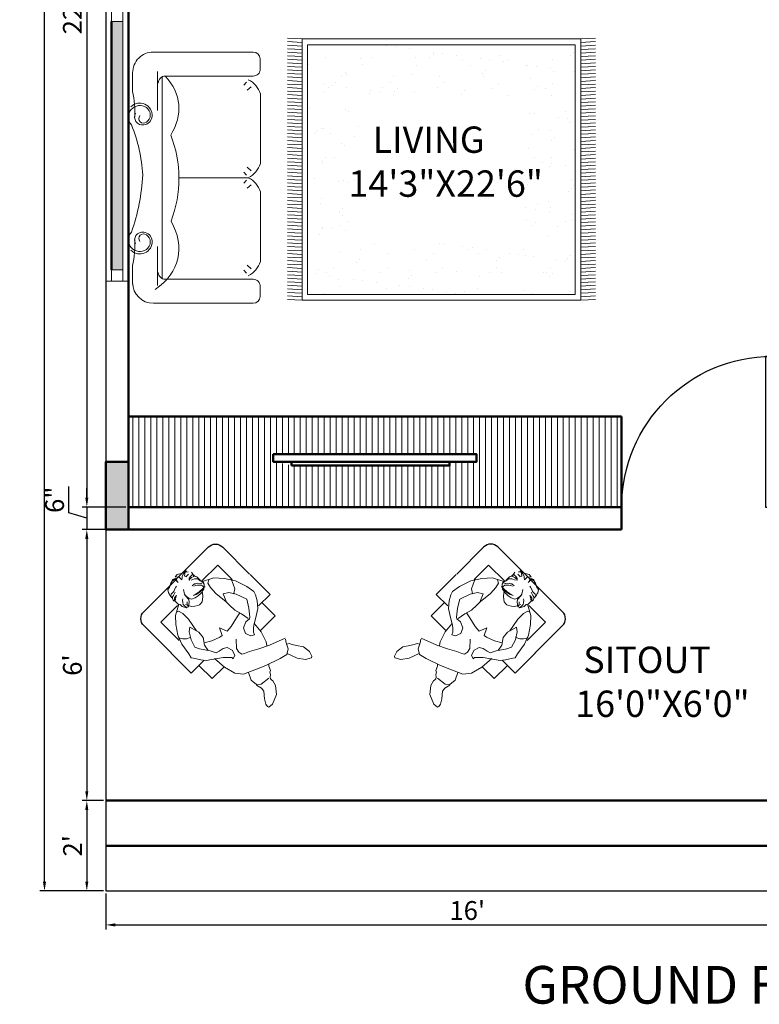
# Model space of a CAD drawing. Units: inches. Extents: x 3064 to 19385, y 846 to 15425.
# Tile 26 of 108: x 4742 to 4938, y 846 to 1108. Entities that reach past the tile are written whole.
import ezdxf

# ---------------------------------------------------------------- set-up
doc = ezdxf.new("R2010")
doc.units = ezdxf.units.IN
for name, color, linetype, lineweight in [('A-ANNO-DIMS', 2, 'Continuous', 18), ('A-ANNO-TEXT', 7, 'Continuous', 25), ('A-AREA-IDEN', 3, 'Continuous', 18), ('A-COLS', 1, 'Continuous', 35), ('A-DOOR', 3, 'Continuous', 25), ('A-FURN', 8, 'Continuous', 18), ('A-FURN-PATT', 252, 'Continuous', 13), ('A-GLAZ', 4, 'Continuous', 18), ('A-WALL', 7, 'Continuous', 50), ('C-PROP', 6, 'Continuous', 25)]:
    doc.layers.add(name, color=color, linetype=linetype, lineweight=lineweight)
doc.layers.add('NOITHAT', color=21, linetype='Continuous')
doc.styles.get("Standard").update_dxf_attribs({"font": 'arial.ttf'})
doc.dimstyles.new('ISO-25', dxfattribs={"dimtxt": 9, "dimasz": 2.5, "dimexe": 1.25, "dimexo": 0.625, "dimtad": 1, "dimdec": 1, "dimlunit": 3, "dimtxsty": 'Standard', "dimcen": 2.5, "dimadec": 0, "dimazin": 0, "dimtfac": 1, "dimtdec": 1, "dimtmove": 0, "dimatfit": 3, "dimfxl": 1, "dimarcsym": 0})

# ---------------------------------------------------------------- blocks, each defined once
blk = doc.blocks.new('*U2')
for p, q in [((0, 0), (0, -6)), ((40, 0), (40, -6))]:
    blk.add_line(p, q)
blk.add_lwpolyline([(0, 0), (0, 40), (1.75, 40), (1.75, 0)], close=True)
blk.add_arc((0, 0), 40, 0, 90)
blk = doc.blocks.new('carpet-9')
at = {"color": 0, "linetype": 'ByBlock'}
for p, q in [((-2.5225, -0.1423), (-2.5308, 0)), ((-2.4883, -0.1423), (-2.4966, 0)), ((-2.4541, -0.1423), (-2.4624, 0)), ((-2.4199, -0.1423), (-2.4282, 0)), ((-2.3857, -0.1423), (-2.394, 0)), ((-2.3515, -0.1423), (-2.3598, 0)), ((-2.3173, -0.1423), (-2.3256, 0)), ((-2.2831, -0.1423), (-2.2914, 0)), ((-2.2489, -0.1423), (-2.2572, 0)), ((-2.2147, -0.1423), (-2.223, 0)), ((-2.1805, -0.1423), (-2.1888, 0)), ((-2.1463, -0.1423), (-2.1546, 0)), ((-2.1121, -0.1423), (-2.1204, 0)), ((-2.0779, -0.1423), (-2.0862, 0)), ((-2.0437, -0.1423), (-2.052, 0)), ((-2.0095, -0.1423), (-2.0178, 0)), ((-1.9753, -0.1423), (-1.9836, 0)), ((-1.9411, -0.1423), (-1.9494, 0)), ((-1.9069, -0.1423), (-1.9152, 0)), ((-1.8727, -0.1423), (-1.881, 0)), ((-1.8385, -0.1423), (-1.8468, 0)), ((-1.8043, -0.1423), (-1.8126, 0)), ((-1.7701, -0.1423), (-1.7784, 0)), ((-1.7359, -0.1423), (-1.7442, 0)), ((-1.7017, -0.1423), (-1.71, 0)), ((-1.6675, -0.1423), (-1.6758, 0)), ((-1.6333, -0.1423), (-1.6416, 0)), ((-1.5991, -0.1423), (-1.6074, 0)), ((-1.5649, -0.1423), (-1.5732, 0)), ((-1.5307, -0.1423), (-1.539, 0)), ((-1.4965, -0.1423), (-1.5048, 0)), ((-1.4623, -0.1423), (-1.4706, 0)), ((-1.4281, -0.1423), (-1.4364, 0)), ((-1.3939, -0.1423), (-1.4022, 0)), ((-1.3597, -0.1423), (-1.368, 0)), ((-1.3255, -0.1423), (-1.3338, 0)), ((-1.2913, -0.1423), (-1.2996, 0)), ((-1.2571, -0.1423), (-1.2654, 0)), ((-1.2229, -0.1423), (-1.2312, 0)), ((-1.1887, -0.1423), (-1.197, 0)), ((-1.1545, -0.1423), (-1.1628, 0)), ((-1.1203, -0.1423), (-1.1286, 0)), ((-1.0861, -0.1423), (-1.0944, 0)), ((-1.0519, -0.1423), (-1.0602, 0)), ((-1.0177, -0.1423), (-1.026, 0)), ((-0.9835, -0.1423), (-0.9918, 0)), ((-0.9493, -0.1423), (-0.9576, 0)), ((-0.9151, -0.1423), (-0.9234, 0)), ((-0.8809, -0.1423), (-0.8892, 0)), ((-0.8467, -0.1423), (-0.855, 0)), ((-0.8125, -0.1423), (-0.8208, 0)), ((-0.7783, -0.1423), (-0.7866, 0)), ((-0.7441, -0.1423), (-0.7524, 0)), ((-0.7099, -0.1423), (-0.7182, 0)), ((-0.6757, -0.1423), (-0.684, 0)), ((-0.6415, -0.1423), (-0.6498, 0)), ((-0.6073, -0.1423), (-0.6156, 0)), ((-0.5731, -0.1423), (-0.5814, 0)), ((-0.5389, -0.1423), (-0.5472, 0)), ((-0.5047, -0.1423), (-0.513, 0)), ((-0.4705, -0.1423), (-0.4788, 0)), ((-0.4363, -0.1423), (-0.4446, 0)), ((-0.4021, -0.1423), (-0.4104, 0)), ((-0.3679, -0.1423), (-0.3762, 0)), ((-0.3337, -0.1423), (-0.342, 0)), ((-0.2995, -0.1423), (-0.3078, 0)), ((-0.2653, -0.1423), (-0.2736, 0)), ((-0.2311, -0.1423), (-0.2394, 0)), ((-0.1969, -0.1423), (-0.2052, 0)), ((-0.1627, -0.1423), (-0.171, 0)), ((-0.1285, -0.1423), (-0.1368, 0)), ((-0.0943, -0.1423), (-0.1026, 0)), ((-0.0601, -0.1423), (-0.0684, 0)), ((-0.0259, -0.1423), (-0.0342, 0)), ((0.0083, -0.1423), (0, 0)), ((0.0081, -0.1423), (-2.5225, -0.1423)), ((-2.5225, -0.1423), (-2.5225, -2.8423)), ((0.0081, -2.8423), (0.0081, -0.1423)), ((-0.0489, -0.1963), (-2.4655, -0.1963)), ((-2.4655, -0.1963), (-2.4655, -2.7883)), ((-2.3955, -0.2124), (-2.3955, -0.2124)), ((-2.3654, -0.2435), (-2.3654, -0.2435)), ((-2.2062, -0.2078), (-2.2062, -0.2078)), ((-1.7544, -0.2756), (-1.7544, -0.2756)), ((-1.7121, -0.2501), (-1.7121, -0.2501)), ((-1.4511, -0.2068), (-1.4511, -0.2068)), ((-1.1533, -0.2312), (-1.1533, -0.2312)), ((-1.1079, -0.2175), (-1.1079, -0.2175)), ((-1.0792, -0.2355), (-1.0792, -0.2355)), ((-1.0491, -0.2666), (-1.0491, -0.2666)), ((-0.8244, -0.2203), (-0.8244, -0.2203)), ((-0.7647, -0.2281), (-0.7647, -0.2281)), ((-0.4215, -0.2387), (-0.4215, -0.2387)), ((-0.3958, -0.2731), (-0.3958, -0.2731)), ((-0.0783, -0.2494), (-0.0783, -0.2494)), ((-0.0489, -2.7883), (-0.0489, -0.1963)), ((-1.8205, -0.2931), (-1.8205, -0.2931)), ((-1.7666, -0.3634), (-1.7666, -0.3634)), ((-1.2958, -0.294), (-1.2958, -0.294)), ((-0.7551, -0.2963), (-0.7551, -0.2963)), ((-0.7072, -0.3675), (-0.7072, -0.3675)), ((-0.3848, -0.3759), (-0.3848, -0.3759)), ((-0.3726, -0.2881), (-0.3726, -0.2881)), ((-2.3219, -0.4132), (-2.3219, -0.4132)), ((-2.2381, -0.437), (-2.2381, -0.437)), ((-2.203, -0.4115), (-2.203, -0.4115)), ((-2.0942, -0.413), (-2.0942, -0.413)), ((-1.9787, -0.4238), (-1.9787, -0.4238)), ((-1.6355, -0.4344), (-1.6355, -0.4344)), ((-1.5701, -0.3969), (-1.5701, -0.3969)), ((-1.54, -0.428), (-1.54, -0.428)), ((-1.3744, -0.4294), (-1.3744, -0.4294)), ((-1.3149, -0.4312), (-1.3149, -0.4312)), ((-1.2923, -0.4451), (-1.2923, -0.4451)), ((-0.949, -0.4557), (-0.949, -0.4557)), ((-0.8867, -0.4345), (-0.8867, -0.4345)), ((-0.8562, -0.4496), (-0.8562, -0.4496)), ((-0.6058, -0.4663), (-0.6058, -0.4663)), ((-0.3091, -0.4326), (-0.3091, -0.4326)), ((-0.2538, -0.4199), (-0.2538, -0.4199)), ((-0.2237, -0.451), (-0.2237, -0.451)), ((-2.061, -0.5583), (-2.061, -0.5583)), ((-2.0464, -0.4841), (-2.0464, -0.4841)), ((-1.6482, -0.5493), (-1.6482, -0.5493)), ((-1.3271, -0.519), (-1.3271, -0.519)), ((-0.9284, -0.5657), (-0.9284, -0.5657)), ((-0.2626, -0.477), (-0.2626, -0.477)), ((-0.2612, -0.5038), (-0.2612, -0.5038)), ((-2.2693, -0.6621), (-2.2693, -0.6621)), ((-2.2571, -0.5742), (-2.2571, -0.5742)), ((-2.1435, -0.6273), (-2.1435, -0.6273)), ((-2.0309, -0.5894), (-2.0309, -0.5894)), ((-1.8003, -0.6379), (-1.8003, -0.6379)), ((-1.7985, -0.5926), (-1.7985, -0.5926)), ((-1.6003, -0.6204), (-1.6003, -0.6204)), ((-1.4571, -0.6486), (-1.4571, -0.6486)), ((-1.3776, -0.5959), (-1.3776, -0.5959)), ((-1.1139, -0.6592), (-1.1139, -0.6592)), ((-0.8753, -0.5867), (-0.8753, -0.5867)), ((-0.7447, -0.5813), (-0.7447, -0.5813)), ((-0.7146, -0.6124), (-0.7146, -0.6124)), ((-0.4167, -0.6051), (-0.4167, -0.6051)), ((-0.0613, -0.619), (-0.0613, -0.619)), ((-2.2675, -0.6823), (-2.2675, -0.6823)), ((-1.2021, -0.6856), (-1.2021, -0.6856)), ((-0.8875, -0.6746), (-0.8875, -0.6746)), ((-0.7706, -0.6698), (-0.7706, -0.6698)), ((-0.4823, -0.702), (-0.4823, -0.702)), ((-0.4357, -0.7423), (-0.4357, -0.7423)), ((-0.4274, -0.6805), (-0.4274, -0.6805)), ((-0.0842, -0.6911), (-0.0842, -0.6911)), ((-2.3197, -0.8449), (-2.3197, -0.8449)), ((-1.9765, -0.8555), (-1.9765, -0.8555)), ((-0.4479, -0.8302), (-0.4479, -0.8302)), ((-2.3593, -0.9188), (-2.3593, -0.9188)), ((-2.3012, -0.8913), (-2.3012, -0.8913)), ((-2.0952, -0.9385), (-2.0952, -0.9385)), ((-0.4101, -0.9272), (-0.4101, -0.9272)), ((-0.2604, -0.9086), (-0.2604, -0.9086)), ((-2.3203, -1.0285), (-2.3203, -1.0285)), ((-2.0474, -1.0097), (-2.0474, -1.0097)), ((-0.3801, -0.9583), (-0.3801, -0.9583)), ((-0.3101, -0.9581), (-0.3101, -0.9581)), ((-0.2622, -1.0293), (-0.2622, -1.0293)), ((-2.3325, -1.1163), (-2.3325, -1.1163)), ((-2.2173, -1.0656), (-2.2173, -1.0656)), ((-2.1872, -1.0967), (-2.1872, -1.0967)), ((-2.1608, -1.0831), (-2.1608, -1.0831)), ((-0.4798, -1.0594), (-0.4798, -1.0594)), ((-0.4448, -1.1362), (-0.4448, -1.1362)), ((-0.2176, -1.1263), (-0.2176, -1.1263)), ((-2.2685, -1.2078), (-2.2685, -1.2078)), ((-0.4989, -1.1966), (-0.4989, -1.1966)), ((-0.4833, -1.2275), (-0.4833, -1.2275)), ((-0.1015, -1.1469), (-0.1015, -1.1469)), ((-2.3257, -1.2866), (-2.3257, -1.2866)), ((-2.0248, -1.2646), (-2.0248, -1.2646)), ((-1.9824, -1.2972), (-1.9824, -1.2972)), ((-0.5111, -1.2844), (-0.5111, -1.2844)), ((-0.0756, -1.2731), (-0.0756, -1.2731)), ((-2.3643, -1.3455), (-2.3643, -1.3455)), ((-0.2664, -1.3504), (-0.2664, -1.3504)), ((-0.0593, -1.3522), (-0.0593, -1.3522)), ((-2.3834, -1.4827), (-2.3834, -1.4827)), ((-2.1587, -1.5148), (-2.1587, -1.5148)), ((-2.0963, -1.464), (-2.0963, -1.464)), ((-0.5429, -1.5136), (-0.5429, -1.5136)), ((-0.5364, -1.4656), (-0.5364, -1.4656)), ((-0.3111, -1.4836), (-0.3111, -1.4836)), ((-0.0715, -1.44), (-0.0715, -1.44)), ((-2.3956, -1.5705), (-2.3956, -1.5705)), ((-2.3737, -1.5729), (-2.3737, -1.5729)), ((-2.3436, -1.604), (-2.3436, -1.604)), ((-2.0484, -1.5352), (-2.0484, -1.5352)), ((-0.4426, -1.5679), (-0.4426, -1.5679)), ((-0.2632, -1.5548), (-0.2632, -1.5548)), ((-0.0994, -1.5785), (-0.0994, -1.5785)), ((-0.3739, -1.6336), (-0.3739, -1.6336)), ((-0.1033, -1.6692), (-0.1033, -1.6692)), ((-2.4274, -1.7997), (-2.4274, -1.7997)), ((-2.343, -1.7423), (-2.343, -1.7423)), ((-2.2695, -1.7333), (-2.2695, -1.7333)), ((-2.1811, -1.7719), (-2.1811, -1.7719)), ((-1.9998, -1.753), (-1.9998, -1.753)), ((-0.4843, -1.753), (-0.4843, -1.753)), ((-0.2837, -1.8061), (-0.2837, -1.8061)), ((-0.2319, -1.7804), (-0.2319, -1.7804)), ((-0.2018, -1.8115), (-0.2018, -1.8115)), ((-0.1224, -1.8064), (-0.1224, -1.8064)), ((-0.1346, -1.8942), (-0.1346, -1.8942)), ((-2.4465, -1.9369), (-2.4465, -1.9369)), ((-2.1646, -1.9565), (-2.1646, -1.9565)), ((-2.0973, -1.9895), (-2.0973, -1.9895)), ((-2.0391, -1.9187), (-2.0391, -1.9187)), ((-2.009, -1.9498), (-2.009, -1.9498)), ((-1.9879, -1.9553), (-1.9879, -1.9553)), ((-2.4587, -2.0248), (-2.4587, -2.0248)), ((-2.0494, -2.0607), (-2.0494, -2.0607)), ((-2.0069, -2.0925), (-2.0069, -2.0925)), ((-0.4485, -2.0096), (-0.4485, -2.0096)), ((-0.3121, -2.0092), (-0.3121, -2.0092)), ((-0.2642, -2.0803), (-0.2642, -2.0803)), ((-0.1053, -2.0203), (-0.1053, -2.0203)), ((-2.3408, -2.174), (-2.3408, -2.174)), ((-2.0191, -2.1804), (-2.0191, -2.1804)), ((-1.9976, -2.1847), (-1.9976, -2.1847)), ((-0.5303, -2.1409), (-0.5303, -2.1409)), ((-0.1665, -2.1234), (-0.1665, -2.1234)), ((-2.3374, -2.2792), (-2.3374, -2.2792)), ((-2.2705, -2.2589), (-2.2705, -2.2589)), ((-0.4854, -2.2785), (-0.4854, -2.2785)), ((-0.3883, -2.2877), (-0.3883, -2.2877)), ((-0.2815, -2.2378), (-0.2815, -2.2378)), ((-0.1855, -2.2606), (-0.1855, -2.2606)), ((-1.6745, -2.2957), (-1.6745, -2.2957)), ((-1.5796, -2.3359), (-1.5796, -2.3359)), ((-1.1573, -2.3333), (-1.1573, -2.3333)), ((-1.0211, -2.3023), (-1.0211, -2.3023)), ((-0.3582, -2.3188), (-0.3582, -2.3188)), ((-0.1977, -2.3485), (-0.1977, -2.3485)), ((-2.1954, -2.426), (-2.1954, -2.426)), ((-2.1819, -2.4122), (-2.1819, -2.4122)), ((-2.1654, -2.4571), (-2.1654, -2.4571)), ((-2.051, -2.4096), (-2.051, -2.4096)), ((-1.8387, -2.4229), (-1.8387, -2.4229)), ((-1.8245, -2.3951), (-1.8245, -2.3951)), ((-1.512, -2.4637), (-1.512, -2.4637)), ((-1.4955, -2.4335), (-1.4955, -2.4335)), ((-1.1523, -2.4441), (-1.1523, -2.4441)), ((-1.1278, -2.4037), (-1.1278, -2.4037)), ((-0.8791, -2.4491), (-0.8791, -2.4491)), ((-0.8091, -2.4548), (-0.8091, -2.4548)), ((-0.7591, -2.3984), (-0.7591, -2.3984)), ((-0.7113, -2.4695), (-0.7113, -2.4695)), ((-0.6692, -2.4221), (-0.6692, -2.4221)), ((-0.4659, -2.4654), (-0.4659, -2.4654)), ((-0.1226, -2.476), (-0.1226, -2.476)), ((-2.0983, -2.515), (-2.0983, -2.515)), ((-2.0701, -2.5468), (-2.0701, -2.5468)), ((-1.6114, -2.5652), (-1.6114, -2.5652)), ((-1.3785, -2.5314), (-1.3785, -2.5314)), ((-1.14, -2.4915), (-1.14, -2.4915)), ((-0.8491, -2.4802), (-0.8491, -2.4802)), ((-0.6882, -2.5593), (-0.6882, -2.5593)), ((-0.3131, -2.5347), (-0.3131, -2.5347)), ((-0.1957, -2.4867), (-0.1957, -2.4867)), ((-2.3468, -2.6157), (-2.3468, -2.6157)), ((-2.0823, -2.6346), (-2.0823, -2.6346)), ((-2.0504, -2.5862), (-2.0504, -2.5862)), ((-2.0035, -2.6264), (-2.0035, -2.6264)), ((-2.0029, -2.6251), (-2.0029, -2.6251)), ((-1.6603, -2.637), (-1.6603, -2.637)), ((-1.6522, -2.6513), (-1.6522, -2.6513)), ((-1.37, -2.6105), (-1.37, -2.6105)), ((-1.3399, -2.6416), (-1.3399, -2.6416)), ((-1.3171, -2.6476), (-1.3171, -2.6476)), ((-0.9739, -2.6583), (-0.9739, -2.6583)), ((-0.9324, -2.6677), (-0.9324, -2.6677)), ((-0.7004, -2.6471), (-0.7004, -2.6471)), ((-0.6866, -2.6481), (-0.6866, -2.6481)), ((-0.6307, -2.6689), (-0.6307, -2.6689)), ((-0.2652, -2.6058), (-0.2652, -2.6058)), ((-0.2296, -2.5777), (-0.2296, -2.5777)), ((-0.0537, -2.6335), (-0.0537, -2.6335)), ((-1.6305, -2.7023), (-1.6305, -2.7023)), ((-1.6044, -2.7225), (-1.6044, -2.7225)), ((-1.1719, -2.7207), (-1.1719, -2.7207)), ((-0.2875, -2.6795), (-0.2875, -2.6795)), ((-0.2487, -2.7149), (-0.2487, -2.7149)), ((-2.5225, -2.8423), (-2.5308, -2.9845)), ((-2.5225, -2.8423), (0.0081, -2.8423)), ((-2.4883, -2.8423), (-2.4966, -2.9845)), ((-2.4655, -2.7883), (-0.0489, -2.7883)), ((-2.4541, -2.8423), (-2.4624, -2.9845)), ((-2.4199, -2.8423), (-2.4282, -2.9845)), ((-2.3857, -2.8423), (-2.394, -2.9845)), ((-2.3515, -2.8423), (-2.3598, -2.9845)), ((-2.3173, -2.8423), (-2.3256, -2.9845)), ((-2.2831, -2.8423), (-2.2914, -2.9845)), ((-2.2715, -2.7844), (-2.2715, -2.7844)), ((-2.2489, -2.8423), (-2.2572, -2.9845)), ((-2.2147, -2.8423), (-2.223, -2.9845)), ((-2.1805, -2.8423), (-2.1888, -2.9845)), ((-2.1463, -2.8423), (-2.1546, -2.9845)), ((-2.1121, -2.8423), (-2.1204, -2.9845)), ((-2.0779, -2.8423), (-2.0862, -2.9845)), ((-2.0437, -2.8423), (-2.052, -2.9845)), ((-2.0095, -2.8423), (-2.0178, -2.9845)), ((-1.9753, -2.8423), (-1.9836, -2.9845)), ((-1.9411, -2.8423), (-1.9494, -2.9845)), ((-1.9069, -2.8423), (-1.9152, -2.9845)), ((-1.8727, -2.8423), (-1.881, -2.9845)), ((-1.8609, -2.7719), (-1.8609, -2.7719)), ((-1.8385, -2.8423), (-1.8468, -2.9845)), ((-1.8043, -2.8423), (-1.8126, -2.9845)), ((-1.7701, -2.8423), (-1.7784, -2.9845)), ((-1.7359, -2.8423), (-1.7442, -2.9845)), ((-1.7017, -2.8423), (-1.71, -2.9845)), ((-1.6675, -2.8423), (-1.6758, -2.9845)), ((-1.6333, -2.8423), (-1.6416, -2.9845)), ((-1.5991, -2.8423), (-1.6074, -2.9845)), ((-1.5649, -2.8423), (-1.5732, -2.9845)), ((-1.5307, -2.8423), (-1.539, -2.9845)), ((-1.4965, -2.8423), (-1.5048, -2.9845)), ((-1.4623, -2.8423), (-1.4706, -2.9845)), ((-1.4281, -2.8423), (-1.4364, -2.9845)), ((-1.3939, -2.8423), (-1.4022, -2.9845)), ((-1.3597, -2.8423), (-1.368, -2.9845)), ((-1.3255, -2.8423), (-1.3338, -2.9845)), ((-1.2913, -2.8423), (-1.2996, -2.9845)), ((-1.2571, -2.8423), (-1.2654, -2.9845)), ((-1.2229, -2.8423), (-1.2312, -2.9845)), ((-1.2062, -2.7876), (-1.2062, -2.7876)), ((-1.1887, -2.8423), (-1.197, -2.9845)), ((-1.1545, -2.8423), (-1.1628, -2.9845)), ((-1.1203, -2.8423), (-1.1286, -2.9845)), ((-1.0861, -2.8423), (-1.0944, -2.9845)), ((-1.0519, -2.8423), (-1.0602, -2.9845)), ((-1.0177, -2.8423), (-1.026, -2.9845)), ((-0.9835, -2.8423), (-0.9918, -2.9845)), ((-0.9493, -2.8423), (-0.9576, -2.9845)), ((-0.9151, -2.8423), (-0.9234, -2.9845)), ((-0.8809, -2.8423), (-0.8892, -2.9845)), ((-0.8467, -2.8423), (-0.855, -2.9845)), ((-0.8125, -2.8423), (-0.8208, -2.9845)), ((-0.7783, -2.8423), (-0.7866, -2.9845)), ((-0.7441, -2.8423), (-0.7524, -2.9845)), ((-0.7099, -2.8423), (-0.7182, -2.9845)), ((-0.6757, -2.8423), (-0.684, -2.9845)), ((-0.6415, -2.8423), (-0.6498, -2.9845)), ((-0.6073, -2.8423), (-0.6156, -2.9845)), ((-0.5731, -2.8423), (-0.5814, -2.9845)), ((-0.5389, -2.8423), (-0.5472, -2.9845)), ((-0.5047, -2.8423), (-0.513, -2.9845)), ((-0.4705, -2.8423), (-0.4788, -2.9845)), ((-0.4363, -2.8423), (-0.4446, -2.9845)), ((-0.4021, -2.8423), (-0.4104, -2.9845)), ((-0.3679, -2.8423), (-0.3762, -2.9845)), ((-0.3337, -2.8423), (-0.342, -2.9845)), ((-0.2995, -2.8423), (-0.3078, -2.9845)), ((-0.2653, -2.8423), (-0.2736, -2.9845)), ((-0.2311, -2.8423), (-0.2394, -2.9845)), ((-0.1969, -2.8423), (-0.2052, -2.9845)), ((-0.1627, -2.8423), (-0.171, -2.9845)), ((-0.1285, -2.8423), (-0.1368, -2.9845)), ((-0.0943, -2.8423), (-0.1026, -2.9845)), ((-0.0601, -2.8423), (-0.0684, -2.9845)), ((-0.0259, -2.8423), (-0.0342, -2.9845)), ((0.0083, -2.8423), (0, -2.9845))]:
    blk.add_line(p, q, dxfattribs=at)
blk = doc.blocks.new('sofa-33')
at = {"color": 0, "linetype": 'ByBlock'}
for p, q in [((-0.15, 0.15), (-0.15, 0.8738)), ((-0.026, 0.9238), (-0.1, 0.9238)), ((0.024, 0.2361), (0.024, 0.8738)), ((0.1006, 0.8574), (0.1265, 0.8286)), ((0.657, 0.9252), (0.1531, 0.9252)), ((0.7096, 0.8574), (0.6837, 0.8286)), ((0.8107, 0.8574), (0.8366, 0.8286)), ((0.8633, 0.9252), (1.3671, 0.9252)), ((1.4197, 0.8574), (1.3938, 0.8286)), ((1.4963, 0.2361), (1.4963, 0.8738)), ((1.6203, 0.9238), (1.5463, 0.9238)), ((1.6703, 0.15), (1.6703, 0.8738)), ((0.05, 0.8375), (0.05, 0.8379)), ((0.0903, 0.8062), (0.0682, 0.8242)), ((0.7199, 0.8062), (0.742, 0.8242)), ((0.7602, 0.8375), (0.7601, 0.8379)), ((0.7601, 0.8375), (0.7601, 0.8379)), ((0.7602, 0.8375), (0.7602, 0.3356)), ((0.8004, 0.8062), (0.7783, 0.8242)), ((1.43, 0.8062), (1.4521, 0.8242)), ((1.4702, 0.8375), (1.4703, 0.8379)), ((1.4702, 0.8375), (1.4703, 0.8379)), ((0.0289, 0.2145), (1.4914, 0.2145)), ((-0.01, 0.1801), (0.2738, 0.1801)), ((1.5422, 0.1801), (1.2585, 0.1801)), ((0, 0), (0.1356, 0)), ((1.5322, 0), (1.3966, 0))]:
    blk.add_line(p, q, dxfattribs=at)
at = {"color": 0, "linetype": 'ByBlock', "extrusion": (0, 0, -1)}
for centre, major_axis, ratio, start_param, end_param in [((-0.1, 0.8738), (0.0354, 0.0354), 1, 3.926992, 5.497787), ((-0.026, 0.8738), (-0.0354, 0.0354), 1, 0.785398, 2.356196), ((0.1997, 0.7661), (0.1173, 0.1173), 1, 4.372209, 5.213218), ((0.6105, 0.7661), (0.1173, 0.1173), 1, -0.500829, 0.34018), ((0.9098, 0.7661), (0.1173, 0.1173), 1, 4.372209, 5.213218), ((1.3206, 0.7661), (-0.1173, 0.1173), 1, 1.069968, 1.910976), ((1.5463, 0.8738), (-0.0354, 0.0354), 1, 5.497786, 7.068583), ((1.6203, 0.8738), (0.0354, 0.0354), 1, -0.785398, 0.785398), ((0.3234, -0.6657), (-0.0931, 0.9998), 0.551284, -0.397889, 0.397889), ((1.147, -0.5336), (0.1998, 0.8608), 0.59532, -0.502747, 0.502747), ((0.7664, -0.6685), (-0.0034, 1.0041), 0.922365, -0.343589, 0.343589), ((0.074, 0.2361), (-0.0354, 0.0354), 1, 3.926991, 5.497788), ((1.4463, 0.2361), (0.0354, 0.0354), 1, 0.785397, 2.356194), ((0, 0.15), (0.1061, 0.1061), 1, 2.356194, 3.926992), ((0.3076, 0.0525), (-0.0624, 0.0624), 1, 4.675944, 7.152385), ((1.2246, 0.0525), (-0.0624, 0.0624), 1, 0.701599, 3.17804), ((1.5203, 0.15), (0.1061, 0.1061), 1, 0.785398, 2.356194), ((0.3208, 0.0524), (-0.059, 0.059), 1, 3.186406, 6.094039), ((0.3052, 0.0629), (-0.0458, 0.0458), 1, 6.094039, 8.043134), ((0.3201, 0.0726), (-0.0414, 0.0414), 1, 2.230507, 4.423483), ((0.3301, 0.0798), (0.0245, 0.0245), 1, 0.189152, 2.952444), ((0.3092, 0.0712), (0.0491, 0.0491), 1, -0.701597, 0.659711), ((0.8779, -1.3822), (-0.3228, 1.4289), 0.878591, -0.144977, 0.144977), ((0.6669, -1.3904), (1.0359, 1.0359), 1, 5.547613, 5.837566), ((1.2122, 0.0726), (-0.0414, 0.0414), 1, 3.430501, 5.623477), ((1.223, 0.0712), (-0.0491, 0.0491), 1, 5.623477, 6.984784), ((1.2115, 0.0524), (0.059, 0.059), 1, 0.189149, 3.096782), ((1.2022, 0.0798), (0.0245, 0.0245), 1, 1.759947, 4.52324), ((1.227, 0.0629), (0.0458, 0.0458), 1, 4.52324, 6.472335), ((0.2824, -0.6613), (-0.479, 0.479), 1, 0.566947, 0.842011), ((1.2498, -0.6613), (0.479, 0.479), 1, 5.441177, 5.716241)]:
    blk.add_ellipse(centre, major_axis=major_axis, ratio=ratio, start_param=start_param, end_param=end_param, dxfattribs=at)
blk = doc.blocks.new('A$C48E80792')
for p, q in [((252, 804.1), (267.8, 807.6)), ((253.5, 801.9), (261.1, 805.7)), ((261.1, 805.7), (274.4, 805.7)), ((267.8, 807.6), (270.5, 811.7)), ((284, 805.7), (270.6, 811.4)), ((274.4, 805.7), (278.3, 805.7)), ((278.3, 805.7), (278.3, 798.1)), ((284, 794.3), (284, 805.7)), ((289.7, 811.4), (305.5, 811.7)), ((289.7, 811.4), (303, 796.2)), ((305.5, 811.7), (317.9, 805.5)), ((317.9, 805.5), (328.1, 800)), ((202, 746.6), (204.7, 764.4)), ((202, 746.6), (205.8, 759.9)), ((204.7, 764.4), (207.4, 769.9)), ((205.8, 759.9), (213.4, 763.8)), ((207.4, 769.9), (208.1, 777.4)), ((208.1, 777.4), (217.7, 791.8)), ((213.4, 763.8), (222.9, 763.8)), ((217.2, 750.4), (226.8, 754.2)), ((217.7, 791.8), (230.8, 792.5)), ((222.9, 763.8), (232.5, 763.8)), ((226.8, 754.2), (234.4, 756.1)), ((230.8, 792.5), (252, 804.1)), ((232.5, 763.8), (236.3, 765.7)), ((236.3, 765.7), (242, 767.6)), ((242, 767.6), (255.4, 771.4)), ((255.4, 771.4), (261.1, 773.3)), ((278.3, 798.1), (280.2, 788.5)), ((280.2, 786.6), (284, 794.3)), ((280.2, 788.5), (280.2, 780.9)), ((280.2, 780.9), (280.2, 786.6)), ((303, 796.2), (303, 779)), ((303, 777.1), (312.6, 782.8)), ((303, 779), (303, 777.1)), ((312.6, 782.8), (318.3, 788.5)), ((318.3, 788.5), (329.8, 792.4)), ((335.5, 786.6), (327.8, 780.9)), ((327.8, 780.9), (327.8, 775.2)), ((327.8, 748.5), (335.5, 756.1)), ((328.1, 800), (343.9, 798)), ((329.8, 792.4), (343.1, 794.3)), ((329.8, 771.4), (335.5, 773.3)), ((343.1, 792.4), (335.5, 786.6)), ((335.5, 773.3), (346.9, 773.3)), ((335.5, 756.1), (346.9, 758)), ((343.1, 794.3), (352.6, 794.3)), ((352.6, 792.4), (343.1, 792.4)), ((343.9, 798), (352.1, 795.9)), ((343.9, 790.4), (354.9, 782.2)), ((346.9, 758), (358.4, 758)), ((358.4, 758), (362.2, 756.1)), ((366, 769.5), (362.2, 750.4)), ((362.2, 756.1), (364.1, 750.4)), ((198.1, 735.2), (202, 742.8)), ((198.1, 727.5), (198.1, 735.2)), ((202, 727.5), (200.1, 725.6)), ((202, 742.8), (207.7, 748.5)), ((211.5, 737.1), (202, 727.5)), ((202, 723.7), (209.6, 729.4)), ((202, 716.1), (202, 723.7)), ((202, 706.6), (202, 716.1)), ((202, 702.8), (202, 706.6)), ((207.7, 748.5), (217.2, 750.4)), ((209.6, 729.4), (219.1, 735.2)), ((219.1, 739), (211.5, 737.1)), ((226.8, 739), (219.1, 739)), ((219.1, 735.2), (226.8, 739)), ((226.8, 739), (226.8, 739)), ((232.5, 700.8), (238.2, 704.7)), ((259.2, 708.5), (257.3, 679.9)), ((260.3, 708.9), (259.6, 699.3)), ((261.6, 715.7), (260.3, 708.9)), ((274, 735.6), (261.6, 715.7)), ((318.3, 718), (333.6, 716.1)), ((331.7, 706.6), (324, 710.4)), ((329.8, 748.5), (327.8, 748.5)), ((335.5, 750.4), (329.8, 748.5)), ((339.3, 700.8), (331.7, 706.6)), ((333.6, 716.1), (339.3, 712.3)), ((337.4, 750.4), (335.5, 750.4)), ((352.6, 735.2), (335.5, 742.8)), ((341.2, 750.4), (337.4, 750.4)), ((339.3, 712.3), (346.9, 708.5)), ((346.9, 750.4), (341.2, 750.4)), ((354.5, 746.6), (346.9, 750.4)), ((346.9, 708.5), (358.4, 695.1)), ((356.5, 731.3), (352.6, 735.2)), ((362.2, 742.8), (354.5, 746.6)), ((362.2, 750.4), (356.5, 746.6)), ((362.2, 723.7), (356.5, 731.3)), ((367.9, 733.3), (362.2, 742.8)), ((364.1, 718), (362.2, 723.7)), ((364.1, 750.4), (364.1, 742.8)), ((364.1, 742.8), (364.1, 739)), ((366, 706.6), (364.1, 718)), ((367.9, 698.9), (366, 706.6)), ((367.9, 706.6), (367.9, 733.3)), ((151.7, 671.2), (119.2, 637.1)), ((204, 699.4), (151.7, 671.2)), ((165.1, 679.5), (178.4, 675)), ((178.4, 675), (185.1, 650.5)), ((207.7, 693.2), (202, 702.8)), ((207.7, 679.9), (207.7, 693.2)), ((219.1, 658.9), (207.7, 679.9)), ((219.1, 681.8), (224.8, 691.3)), ((219.1, 670.3), (219.1, 681.8)), ((221, 657), (219.1, 670.3)), ((224.8, 691.3), (232.5, 700.8)), ((226.8, 655.1), (232.5, 664.6)), ((232.5, 657), (226.8, 655.1)), ((227.3, 673.2), (235.6, 655.4)), ((232.5, 664.6), (236.3, 670.3)), ((238.2, 660.8), (232.5, 657)), ((235.6, 655.4), (243.8, 644.4)), ((236.3, 670.3), (243.9, 678)), ((249.6, 670.3), (238.2, 660.8)), ((257.3, 679.9), (249.6, 670.3)), ((259.6, 699.3), (261.6, 685.6)), ((261.6, 685.6), (269.2, 671.8)), ((269.2, 671.8), (285.6, 662.9)), ((285.6, 662.9), (304.8, 659.5)), ((302.1, 672.5), (287, 679.4)), ((287, 679.4), (304.8, 673.9)), ((323.3, 667), (302.1, 672.5)), ((304.8, 673.9), (323.3, 670.5)), ((304.8, 659.5), (326.8, 659.5)), ((319.2, 640.3), (330.9, 654)), ((323.3, 670.5), (345.3, 668.4)), ((337.7, 666.4), (323.3, 667)), ((326.8, 659.5), (340.5, 661.6)), ((330.9, 654), (334, 660.6)), ((356.3, 669.8), (337.7, 666.4)), ((346.9, 693.2), (339.3, 700.8)), ((340.5, 661.6), (348.7, 664.3)), ((345.3, 668.4), (356.3, 668.4)), ((354.5, 685.6), (346.9, 693.2)), ((348.7, 664.3), (352.1, 667.7)), ((352.1, 667.7), (356.3, 669.8)), ((356.5, 676.1), (354.5, 685.6)), ((356.3, 668.4), (367.2, 680.1)), ((356.3, 668.4), (358.3, 669.8)), ((362.2, 666.5), (356.5, 676.1)), ((358.4, 695.1), (360.3, 693.2)), ((360.3, 693.2), (366, 691.3)), ((366, 691.3), (369.8, 689.4)), ((366.5, 698.9), (425.1, 668)), ((367.2, 680.1), (370.7, 689)), ((371.7, 691.3), (367.9, 698.9)), ((369.8, 689.4), (371.7, 689.4)), ((371.7, 689.4), (371.7, 691.3)), ((371.7, 689.4), (371.7, 689.4)), ((385.6, 670.5), (378.9, 646.1)), ((401.2, 679.5), (385.6, 670.5)), ((425.1, 668), (462.5, 627.3)), ((119.2, 637.1), (88.2, 591.5)), ((185.1, 610.4), (178.4, 572.6)), ((185.1, 650.5), (185.1, 610.4)), ((243.8, 644.4), (254.8, 633.5)), ((254.8, 633.5), (267.8, 625.9)), ((267.8, 625.9), (276.7, 622.5)), ((276.7, 622.5), (283.6, 621.8)), ((283.6, 621.8), (298, 623.9)), ((298, 623.9), (307.6, 630.7)), ((307.6, 630.7), (319.2, 640.3)), ((378.9, 646.1), (376.7, 603.8)), ((376.7, 603.8), (383.3, 537)), ((462.5, 627.3), (493.4, 580.1)), ((485.8, 606), (472.4, 574.8)), ((88.2, 591.5), (70.3, 544.3)), ((80.4, 579.3), (93.8, 559.2)), ((93.8, 559.2), (107.1, 545.9)), ((119.2, 526.5), (141.9, 562.2)), ((141.9, 562.2), (161.5, 576.9)), ((161.5, 576.9), (175.7, 525.7)), ((178.4, 572.6), (171.7, 539.2)), ((402.3, 576.9), (383.3, 535)), ((426.7, 560.6), (402.3, 576.9)), ((447.9, 528.1), (426.7, 560.6)), ((472.4, 574.8), (461.3, 552.6)), ((493.4, 580.1), (513, 518.3)), ((70.3, 544.3), (60.6, 484.2)), ((106.8, 485.6), (119.2, 526.5)), ((107.1, 545.9), (125, 539.2)), ((125, 539.2), (129.4, 537)), ((175.7, 525.7), (172, 490.5)), ((383.3, 535), (383.3, 512.7)), ((383.3, 512.7), (385.2, 475.7)), ((461.3, 552.6), (441.3, 539.2)), ((441.3, 539.2), (441.3, 537)), ((467.4, 472.8), (447.9, 528.1)), ((513, 518.3), (521.1, 474.4)), ((60.6, 484.2), (55.7, 461.4)), ((55.7, 461.4), (62.2, 451.6)), ((117.5, 463), (106.8, 485.6)), ((149.1, 418.9), (117.5, 463)), ((149.7, 459), (143.7, 426.5)), ((172, 490.5), (149.7, 459)), ((156.1, 468), (191.8, 447.9)), ((247.5, 430.1), (265.3, 468)), ((265.3, 468), (276.4, 439)), ((385.2, 475.7), (396.3, 438.6)), ((443, 432.1), (467.4, 472.8)), ((514.6, 456.5), (499.9, 428.9)), ((521.1, 474.4), (514.6, 456.5)), ((62.2, 451.6), (81.7, 419.1)), ((81.7, 419.1), (99.6, 398)), ((163.7, 389.7), (149.1, 418.9)), ((191.8, 447.9), (234.1, 432.3)), ((234.1, 432.3), (247.5, 430.1)), ((276.4, 439), (280.9, 427.9)), ((280.9, 427.9), (312.1, 430.1)), ((312.1, 430.1), (363.3, 441.2)), ((363.3, 441.2), (392.3, 447.9)), ((396.3, 438.6), (403.7, 397.8)), ((413.7, 396.3), (443, 432.1)), ((499.9, 428.9), (473.9, 399.6)), ((99.6, 398), (147.5, 363.6)), ((136.8, 373.8), (142.3, 307)), ((147.5, 363.6), (171.9, 347.4)), ((180, 384.8), (163.7, 389.7)), ((204.4, 379.9), (180, 384.8)), ((222.3, 368.5), (204.4, 379.9)), ((230.5, 340.9), (222.3, 368.5)), ((285.1, 367.1), (252.6, 331.3)), ((338.8, 352.4), (351.9, 380.1)), ((350.2, 324.8), (338.8, 352.4)), ((351.9, 380.1), (382.8, 393.1)), ((382.8, 393.1), (405.6, 391.5)), ((405.6, 355.7), (389.3, 345.9)), ((407.4, 355.2), (401.9, 303.3)), ((405.6, 391.5), (413.7, 396.3)), ((433.2, 373.6), (405.6, 355.7)), ((473.9, 399.6), (433.2, 373.6)), ((142.3, 307), (157.1, 247.7)), ((171.9, 347.4), (191.4, 326.2)), ((191.4, 326.2), (202.8, 314.8)), ((202.8, 314.8), (202.8, 306.7)), ((202.8, 306.7), (222.3, 313.2)), ((222.3, 313.2), (230.5, 340.9)), ((252.6, 331.3), (247.7, 310.1)), ((247.7, 310.1), (251, 292.3)), ((366.5, 315), (350.2, 324.8)), ((373, 329.7), (366.5, 315)), ((389.3, 345.9), (373, 329.7)), ((401.9, 303.3), (383.3, 247.7)), ((251, 292.3), (262.4, 284.1)), ((262.4, 284.1), (288.4, 272.7)), ((288.4, 272.7), (332.3, 250)), ((157.1, 247.7), (185, 214.4)), ((185, 214.4), (249.8, 184.7)), ((209.1, 201.4), (190.5, 164.4)), ((332.3, 250), (384.4, 223.9)), ((383.3, 247.7), (372.2, 232.9)), ((384.4, 223.9), (466, 193.4)), ((190.5, 164.4), (194.2, 129.2)), ((249.8, 184.7), (296.2, 164.4)), ((295.8, 130.1), (305.5, 151.4)), ((296.2, 164.4), (374.1, 136.6)), ((305.5, 151.4), (311, 157)), ((437.1, 144), (452.7, 171.9)), ((461.2, 158.8), (450.1, 164.4)), ((452.7, 171.9), (462.5, 188.2)), ((468.1, 144.2), (461.2, 158.8)), ((192.4, 126.7), (199, 98.4)), ((194.2, 129.2), (212.8, 112.5)), ((212.8, 112.5), (261.8, 106.9)), ((265.8, 98.4), (270.8, 106.7)), ((270.8, 106.7), (280.8, 115.1)), ((280.8, 115.1), (287.5, 125.1)), ((287.5, 125.1), (295.8, 130.1)), ((374.1, 136.6), (413, 127.3)), ((413, 127.3), (437.1, 144)), ((417.2, 129.7), (436.8, 77.9)), ((480.4, 126.2), (468.1, 144.2)), ((500.2, 94.8), (480.4, 126.2)), ((197.4, 78.4), (170.7, 48.4)), ((199, 98.4), (197.4, 78.4)), ((230.7, 21.7), (259.1, 56.7)), ((259.1, 56.7), (265.8, 83.4)), ((265.8, 91.7), (265.8, 98.4)), ((265.8, 83.4), (265.8, 91.7)), ((436.8, 77.9), (461.5, 41.9)), ((496.7, 31.6), (505.1, 56.7)), ((505.1, 56.7), (500.2, 94.8)), ((157.3, 25), (154, 10)), ((154, 10), (157.3, 1.7)), ((170.7, 48.4), (157.3, 25)), ((157.3, 1.7), (180.7, 0)), ((180.7, 0), (230.7, 21.7)), ((461.5, 41.9), (488.5, 26.9)), ((488.5, 26.9), (496.7, 31.6))]:
    blk.add_line(p, q)
blk.add_arc((337.3, 639.4), 150, 89.3152, 90)
at = {"layer": 'NOITHAT'}
for p, q in [((0.2, 550.4), (0, 405.9)), ((569, 405.9), (569.1, 549.9))]:
    blk.add_line(p, q, dxfattribs=at)
blk.add_lwpolyline([(0.1, 548.9), (0.1, 748.9, -0.414214), (50.1, 798.9), (518.1, 798.9, -0.414214), (568.1, 748.9), (568.1, 551.9)], format="xyb", dxfattribs=at)
for points in [[(195.1, 699.9), (74.1, 699.9), (74.1, 567.9)], [(486.1, 596.9), (486.1, 699.9), (369.1, 699.9)], [(92.1, 405.9), (0, 405.9)], [(56.1, 405.9), (56.1, 309.9), (142.1, 309.9)], [(402.6, 309.9), (510.1, 309.9), (510.1, 405.9)], [(486.1, 405.9), (569, 405.9)]]:
    blk.add_lwpolyline(points, dxfattribs=at)
blk = doc.blocks.new('*D51')
at = {"layer": 'A-ANNO-DIMS', "color": 0, "lineweight": -2, "transparency": 16777216}
for p, q in [((4763.85, 1248.1), (4758.2, 1248.1)), ((4759.45, 1245.6), (4759.45, 980.6)), ((4769.85, 978.1), (4758.2, 978.1))]:
    blk.add_line(p, q, dxfattribs=at)
at = {"layer": 'A-ANNO-DIMS', "color": 0, "transparency": 16777216}
for points in [[(4759.03, 1245.6), (4759.86, 1245.6), (4759.45, 1248.1)], [(4759.03, 980.6), (4759.86, 980.6), (4759.45, 978.1)]]:
    blk.add_solid(points, dxfattribs=at)
at = {"layer": 'Defpoints', "color": 0, "transparency": 16777216}
for p in [(4764.48, 1248.1), (4759.45, 978.1), (4770.48, 978.1)]:
    blk.add_point(p, dxfattribs=at)
at = {"layer": 'A-ANNO-DIMS', "color": 0, "transparency": 16777216, "insert": (4756.27, 1113.1), "char_height": 5, "attachment_point": 5, "rotation": 90}
blk.add_mtext('22\'-6"', dxfattribs=at)
blk = doc.blocks.new('*D52')
at = {"layer": 'A-ANNO-DIMS', "color": 0, "lineweight": -2, "transparency": 16777216}
for p, q in [((4754.71, 976.52), (4754.71, 983.54)), ((4759.45, 980.6), (4759.45, 983.1)), ((4759.45, 975.1), (4754.71, 976.52)), ((4769.85, 978.1), (4758.2, 978.1)), ((4759.45, 978.1), (4759.45, 972.1)), ((4759.45, 978.1), (4759.45, 972.1)), ((4769.85, 972.1), (4758.2, 972.1)), ((4759.45, 969.6), (4759.45, 967.1))]:
    blk.add_line(p, q, dxfattribs=at)
at = {"layer": 'A-ANNO-DIMS', "color": 0, "transparency": 16777216}
for points in [[(4759.03, 980.6), (4759.86, 980.6), (4759.45, 978.1)], [(4759.03, 969.6), (4759.86, 969.6), (4759.45, 972.1)]]:
    blk.add_solid(points, dxfattribs=at)
at = {"layer": 'Defpoints', "color": 0, "transparency": 16777216}
for p in [(4770.48, 978.1), (4759.45, 972.1), (4770.48, 972.1)]:
    blk.add_point(p, dxfattribs=at)
at = {"layer": 'A-ANNO-DIMS', "color": 0, "transparency": 16777216, "insert": (4751.53, 980.03), "char_height": 5, "attachment_point": 5, "rotation": 90}
blk.add_mtext('6"', dxfattribs=at)
blk = doc.blocks.new('*D53')
at = {"layer": 'A-ANNO-DIMS', "color": 0, "lineweight": -2, "transparency": 16777216}
for p, q in [((4769.85, 972.1), (4758.2, 972.1)), ((4759.45, 969.6), (4759.45, 902.6)), ((4763.85, 900.1), (4758.2, 900.1))]:
    blk.add_line(p, q, dxfattribs=at)
at = {"layer": 'A-ANNO-DIMS', "color": 0, "transparency": 16777216}
for points in [[(4759.03, 969.6), (4759.86, 969.6), (4759.45, 972.1)], [(4759.03, 902.6), (4759.86, 902.6), (4759.45, 900.1)]]:
    blk.add_solid(points, dxfattribs=at)
at = {"layer": 'Defpoints', "color": 0, "transparency": 16777216}
for p in [(4770.48, 972.1), (4759.45, 900.1), (4764.48, 900.1)]:
    blk.add_point(p, dxfattribs=at)
at = {"layer": 'A-ANNO-DIMS', "color": 0, "transparency": 16777216, "insert": (4756.27, 936.1), "char_height": 5, "attachment_point": 5, "rotation": 90}
blk.add_mtext("6'", dxfattribs=at)
blk = doc.blocks.new('*D54')
at = {"layer": 'A-ANNO-DIMS', "color": 0, "lineweight": -2, "transparency": 16777216}
for p, q in [((4763.85, 900.1), (4758.2, 900.1)), ((4759.45, 897.6), (4759.45, 878.6)), ((4763.85, 876.1), (4758.2, 876.1))]:
    blk.add_line(p, q, dxfattribs=at)
at = {"layer": 'A-ANNO-DIMS', "color": 0, "transparency": 16777216}
for points in [[(4759.03, 897.6), (4759.86, 897.6), (4759.45, 900.1)], [(4759.03, 878.6), (4759.86, 878.6), (4759.45, 876.1)]]:
    blk.add_solid(points, dxfattribs=at)
at = {"layer": 'Defpoints', "color": 0, "transparency": 16777216}
for p in [(4764.48, 900.1), (4759.45, 876.1), (4764.48, 876.1)]:
    blk.add_point(p, dxfattribs=at)
at = {"layer": 'A-ANNO-DIMS', "color": 0, "transparency": 16777216, "insert": (4756.31, 888.1), "char_height": 5, "attachment_point": 5, "rotation": 90}
blk.add_mtext("2'", dxfattribs=at)
blk = doc.blocks.new('*D55')
at = {"layer": 'A-ANNO-DIMS', "color": 0, "lineweight": -2, "transparency": 16777216}
for p, q in [((4763.85, 1392.1), (4746.96, 1392.1)), ((4748.21, 878.6), (4748.21, 1389.6)), ((4763.85, 876.1), (4746.96, 876.1))]:
    blk.add_line(p, q, dxfattribs=at)
at = {"layer": 'A-ANNO-DIMS', "color": 0, "transparency": 16777216}
for points in [[(4747.79, 1389.6), (4748.63, 1389.6), (4748.21, 1392.1)], [(4747.79, 878.6), (4748.63, 878.6), (4748.21, 876.1)]]:
    blk.add_solid(points, dxfattribs=at)
at = {"layer": 'Defpoints', "color": 0, "transparency": 16777216}
for p in [(4748.21, 1392.1), (4764.48, 1392.1), (4764.48, 876.1)]:
    blk.add_point(p, dxfattribs=at)
at = {"layer": 'A-ANNO-DIMS', "color": 0, "transparency": 16777216, "insert": (4745.03, 1134.1), "char_height": 5, "attachment_point": 5, "rotation": 90}
blk.add_mtext("43'", dxfattribs=at)
blk = doc.blocks.new('*D56')
at = {"layer": 'A-ANNO-DIMS', "color": 0, "lineweight": -2, "transparency": 16777216}
for p, q in [((4764.48, 875.47), (4764.48, 865.83)), ((4956.48, 875.47), (4956.48, 865.83)), ((4766.98, 867.08), (4953.98, 867.08))]:
    blk.add_line(p, q, dxfattribs=at)
at = {"layer": 'A-ANNO-DIMS', "color": 0, "transparency": 16777216}
for points in [[(4766.98, 867.5), (4766.98, 866.67), (4764.48, 867.08)], [(4953.98, 867.5), (4953.98, 866.67), (4956.48, 867.08)]]:
    blk.add_solid(points, dxfattribs=at)
at = {"layer": 'Defpoints', "color": 0, "transparency": 16777216}
for p in [(4764.48, 876.1), (4956.48, 876.1), (4956.48, 867.08)]:
    blk.add_point(p, dxfattribs=at)
at = {"layer": 'A-ANNO-DIMS', "color": 0, "transparency": 16777216, "insert": (4860.48, 870.26), "char_height": 5, "attachment_point": 5}
blk.add_mtext("16'", dxfattribs=at)
blk = doc.blocks.new('WIN-1900')
blk.add_line((3, 0), (3, 66))
blk.add_lwpolyline([(3, 66), (0, 66), (0, 69), (3, 69)], close=True)

msp = doc.modelspace()

# ---------------------------------------------------------------- hatches: boundary and pattern name
at = {"layer": 'A-COLS'}
h = msp.add_hatch(color=256, dxfattribs=at)
h.dxf.hatch_style = 1
h.paths.add_polyline_path([(4770.48, 972.1), (4770.48, 990.1), (4764.48, 990.1), (4764.48, 972.1)])
at = {"layer": 'A-FURN-PATT'}
h = msp.add_hatch(dxfattribs=at)
h.set_pattern_fill('ANSI31', color=256, scale=0.5, angle=45)
h.set_pattern_definition([(90, (-551.1915, -4.2436), (-1.5875, 0), [])])
h.paths.add_polyline_path([(4901.48, 978.1), (4901.48, 1002.1), (4770.48, 1002.1), (4770.48, 978.1)])
h.paths.add_polyline_path([(4862.98, 990.12), (4855.8, 990.12), (4855.8, 989.12), (4813.8, 989.12), (4808.98, 990.12), (4808.98, 992.12), (4862.98, 992.12)], flags=16)
at = {"layer": 'A-GLAZ'}
h = msp.add_hatch(color=256, dxfattribs=at)
h.dxf.hatch_style = 1
h.paths.add_polyline_path([(4765.98, 1041.1), (4768.98, 1041.1), (4768.98, 1107.1), (4765.98, 1107.1)])

# ---------------------------------------------------------------- linework, layer by layer
msp.add_line((4770.48, 1038.1), (4764.48, 1038.1), dxfattribs=at)
msp.add_lwpolyline([(4768.98, 1038.1), (4765.98, 1038.1), (4765.98, 1041.1), (4768.98, 1041.1)], close=True, dxfattribs=at)
at = {"layer": 'A-WALL'}
for p, q in [((4770.48, 1386.1), (4770.48, 978.1)), ((4765.98, 1041.1), (4765.98, 1107.1)), ((4901.48, 1002.1), (4770.48, 1002.1)), ((4901.48, 972.1), (4901.48, 1002.1)), ((4901.48, 978.1), (4770.48, 978.1)), ((4901.48, 972.1), (4764.48, 972.1)), ((4764.48, 900.1), (4956.48, 900.1)), ((4764.48, 888.1), (4956.48, 888.1))]:
    msp.add_line(p, q, dxfattribs=at)
for points in [[(4808.98, 992.12), (4862.98, 992.12), (4862.98, 990.12), (4808.98, 990.12)], [(4770.48, 972.1), (4770.48, 990.1), (4764.48, 990.1), (4764.48, 972.1)], [(4813.8, 989.12), (4855.8, 989.12), (4855.8, 990.12), (4813.8, 990.12)]]:
    msp.add_lwpolyline(points, close=True, dxfattribs=at)
at = {"layer": 'C-PROP'}
for p, q in [((4764.48, 1392.1), (4764.48, 876.1)), ((4764.48, 876.1), (5106.48, 876.1))]:
    msp.add_line(p, q, dxfattribs=at)

# ---------------------------------------------------------------- block references
at = {"layer": 'A-DOOR', "xscale": -1}
msp.add_blockref('*U2', (4941.48, 978.1), dxfattribs=at)
at = {"layer": 'A-FURN'}
for name, p, xscale, yscale, zscale, rotation in [('carpet-9', (4894.57, 1033.24), 27.43020644299853, 27.43020644299853, 27.43020644299853, 270), ('sofa-33', (4771.62, 1093.45), 36.66436083614781, 36.66436083614781, 36.66436083614781, 270), ('A$C48E80792', (4802.1, 919.04), 0.0520199143446925, 0.0520199143446925, 0.0520199143446925, 45.00000000000001), ('A$C48E80792', (4858.27, 919.04), -0.0520199143446925, 0.0520199143446925, 0.0520199143446925, 315)]:
    msp.add_blockref(name, p, dxfattribs=dict(at, xscale=xscale, yscale=yscale, zscale=zscale, rotation=rotation))
at = {"layer": 'A-GLAZ'}
msp.add_blockref('WIN-1900', (4765.98, 1041.1), dxfattribs=at)

# ---------------------------------------------------------------- texts
at = {"layer": 'A-ANNO-TEXT', "insert": (4875.14, 856.17), "char_height": 10, "attachment_point": 1}
msp.add_mtext_dynamic_manual_height_columns('GROUND FLOOR PLAN', width=200.9739, gutter_width=12.5, heights=[0], dxfattribs=at)
at = {"layer": 'A-AREA-IDEN', "char_height": 7, "attachment_point": 1}
for s, insert in [('   LIVING\\P14\'3"X22\'6"', (4828.93, 1079.18)), (' SITOUT\\P16\'0"X6\'0"', (4889.14, 941))]:
    msp.add_mtext_dynamic_manual_height_columns(s, width=67.5924, gutter_width=12.5, heights=[0], dxfattribs=dict(at, insert=insert))

# ---------------------------------------------------------------- dimensions: what is measured, and where the dimension line sits
at = {"layer": 'A-ANNO-DIMS'}
for base, p1, p2, override, picture, middle in [((4748.21, 1392.1), (4764.48, 876.1), (4764.48, 1392.1), {"dimtxt": 5, "dimclrd": 0, "dimclre": 0, "dimclrt": 0}, '*D55', (4745.03, 1134.1)), ((4759.45, 978.1), (4764.48, 1248.1), (4770.48, 978.1), {"dimtxt": 5, "dimclrd": 0, "dimclre": 0, "dimclrt": 0, "dimtmove": 1}, '*D51', (4756.27, 1113.1)), ((4759.45, 972.1), (4770.48, 978.1), (4770.48, 972.1), {"dimtxt": 5, "dimclrd": 0, "dimclre": 0, "dimclrt": 0, "dimtmove": 1}, '*D52', (4751.53, 977.14)), ((4759.45, 900.1), (4770.48, 972.1), (4764.48, 900.1), {"dimtxt": 5, "dimclrd": 0, "dimclre": 0, "dimclrt": 0, "dimtmove": 1}, '*D53', (4756.27, 936.1)), ((4759.45, 876.1), (4764.48, 900.1), (4764.48, 876.1), {"dimtxt": 5, "dimclrd": 0, "dimclre": 0, "dimclrt": 0, "dimtmove": 1}, '*D54', (4756.31, 888.1))]:
    dim = msp.add_linear_dim(base=base, p1=p1, p2=p2, angle=90, dimstyle='ISO-25', override=override, dxfattribs=at)
    dim.commit()
    dim.dimension.update_dxf_attribs({"geometry": picture, "text_midpoint": middle})
dim = msp.add_linear_dim(base=(4956.48, 867.08), p1=(4764.48, 876.1), p2=(4956.48, 876.1), dimstyle='ISO-25', override={"dimtxt": 5, "dimclrd": 0, "dimclre": 0, "dimclrt": 0}, dxfattribs=at)
dim.commit()
dim.dimension.update_dxf_attribs({"geometry": '*D56', "text_midpoint": (4860.48, 870.26)})

doc.saveas('drawing.dxf')
